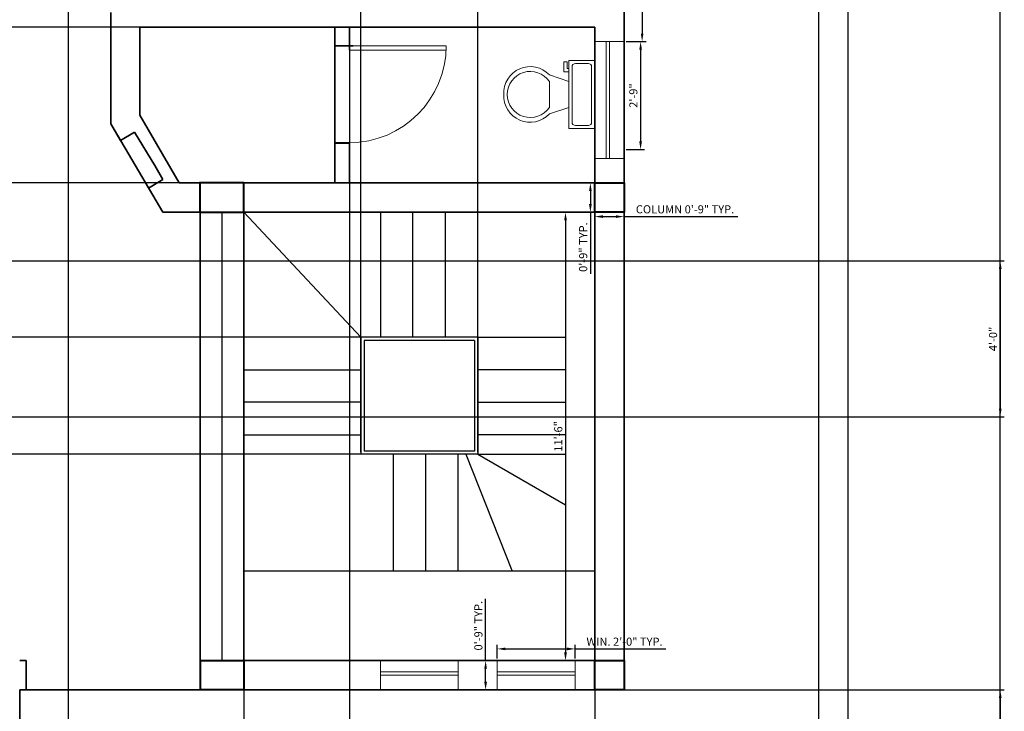
# Model space of a CAD drawing. Units: inches. Extents: x 1624 to 3956, y 1589 to 5028.
# Tile 3 of 16: x 1915 to 2218, y 1862 to 2075. Entities that reach past the tile are written whole.
import ezdxf

# ---------------------------------------------------------------- set-up
doc = ezdxf.new("R2010")
doc.units = ezdxf.units.IN
for name, color, linetype, lineweight in [('A-ANNO-DIMS', 2, 'Continuous', 13), ('A-COLS', 1, 'Continuous', 40), ('A-DOOR', 3, 'Continuous', 18), ('A-FLOR-FIXT', 9, 'Continuous', 18), ('A-FLOR-STRS', 7, 'Continuous', 25), ('A-GLAZ', 4, 'Continuous', 18), ('A-WALL', 7, 'Continuous', 35), ('C-PROP', 7, 'Continuous', 25)]:
    doc.layers.add(name, color=color, linetype=linetype, lineweight=lineweight)
doc.styles.get("Standard").update_dxf_attribs({"font": 'arial.ttf'})
doc.dimstyles.new('Copy of ISO-25', dxfattribs={"dimtxt": 2.5, "dimasz": 2.5, "dimexe": 1.25, "dimexo": 0.625, "dimtad": 1, "dimdec": 1, "dimlunit": 4, "dimtxsty": 'Standard', "dimcen": 2.5, "dimadec": 0, "dimazin": 0, "dimtfac": 1, "dimtdec": 1, "dimtmove": 0, "dimatfit": 3, "dimfxl": 1, "dimarcsym": 0})

# ---------------------------------------------------------------- blocks, each defined once
blk = doc.blocks.new('*D1')
at = {"layer": 'A-ANNO-DIMS', "color": 0, "lineweight": -2, "transparency": 16777216}
for p, q in [((2090.95, 2015.79), (2081.32, 2015.79)), ((2082.57, 2013.29), (2082.57, 1880.29)), ((2090.95, 1877.79), (2081.32, 1877.79))]:
    blk.add_line(p, q, dxfattribs=at)
at = {"layer": 'A-ANNO-DIMS', "color": 0, "transparency": 16777216}
for points in [[(2082.15, 2013.29), (2082.99, 2013.29), (2082.57, 2015.79)], [(2082.15, 1880.29), (2082.99, 1880.29), (2082.57, 1877.79)]]:
    blk.add_solid(points, dxfattribs=at)
at = {"layer": 'Defpoints', "color": 0, "transparency": 16777216}
for p in [(2091.58, 2015.79), (2082.57, 1877.79), (2091.58, 1877.79)]:
    blk.add_point(p, dxfattribs=at)
at = {"layer": 'A-ANNO-DIMS', "color": 0, "transparency": 16777216, "insert": (2080.67, 1946.79), "char_height": 2.5, "attachment_point": 5, "rotation": 90}
blk.add_mtext('11\'-6"', dxfattribs=at)
blk = doc.blocks.new('*U7')
for p, q in [((-40, 0), (-40, 6)), ((0, 0), (0, 6))]:
    blk.add_line(p, q)
blk.add_lwpolyline([(0, 0), (0, -40), (-1.75, -40), (-1.75, 0)], close=True)
blk.add_arc((0, 0), 40, 180, 270)
blk = doc.blocks.new('*U14')
for p, q in [((241.3, -152.4), (241.3, -50.8)), ((-254, -215.9), (-203.2, -215.9)), ((-254, -241.3), (-254, -215.9)), ((-203.2, -215.9), (-203.2, -203.2)), ((-177.8, -203.2), (-177.8, -241.3)), ((-101.6, -203.2), (-152.4, -355.6)), ((101.6, -203.2), (152.4, -355.6)), ((-177.8, -241.3), (-254, -241.3)), ((101.6, -355.6), (-101.6, -355.6))]:
    blk.add_line(p, q)
blk.add_lwpolyline([(266.7, -203.2), (266.7, 0), (-266.7, 0), (-266.7, -203.2)], close=True)
for points in [[(-241.3, -50.8), (-241.3, -152.4)], [(215.9, -25.4), (-215.9, -25.4)], [(-215.9, -177.8), (215.9, -177.8)]]:
    blk.add_lwpolyline(points)
for centre, radius, start, end in [((-219.075, -47.625), 22.45064, 81.8699, 188.1301), ((219.075, -47.625), 22.45064, 351.8699, 98.1301), ((-219.075, -155.575), 22.45064, 171.869898, 278.1301), ((219.075, -155.575), 22.45064, 261.8699, 8.1301), ((-12.12088, -505.93752), 205.61935, 133.01722, 273.38), ((0.94996, -504.77674), 181.02486, 124.50543, 269.7), ((-0.94742, -504.77674), 181.02486, 270.3, 55.4946), ((12.12342, -505.93752), 205.61935, 266.62, 46.9828)]:
    blk.add_arc(centre, radius, start, end)
blk = doc.blocks.new('*D41')
at = {"layer": 'A-ANNO-DIMS', "color": 0, "lineweight": -2, "transparency": 16777216}
for p, q in [((2101.2, 2104.79), (2107.41, 2104.79)), ((2106.16, 2102.29), (2106.16, 2070.79)), ((2101.2, 2068.29), (2107.41, 2068.29))]:
    blk.add_line(p, q, dxfattribs=at)
at = {"layer": 'A-ANNO-DIMS', "color": 0, "transparency": 16777216}
for points in [[(2105.74, 2102.29), (2106.57, 2102.29), (2106.16, 2104.79)], [(2105.74, 2070.79), (2106.57, 2070.79), (2106.16, 2068.29)]]:
    blk.add_solid(points, dxfattribs=at)
at = {"layer": 'Defpoints', "color": 0, "transparency": 16777216}
for p in [(2100.58, 2104.79), (2100.58, 2068.29), (2106.16, 2068.29)]:
    blk.add_point(p, dxfattribs=at)
at = {"layer": 'A-ANNO-DIMS', "color": 0, "transparency": 16777216, "insert": (2102.58, 2086.54), "char_height": 2.5, "attachment_point": 5, "rotation": 90}
blk.add_mtext('3\'-0{\\H1x;\\S1/2;}"', dxfattribs=at)
blk = doc.blocks.new('*D42')
at = {"layer": 'A-ANNO-DIMS', "color": 0, "lineweight": -2, "transparency": 16777216}
for p, q in [((2101.2, 2068.29), (2106.93, 2068.29)), ((2105.68, 2065.79), (2105.68, 2037.58)), ((2101.2, 2035.08), (2106.93, 2035.08))]:
    blk.add_line(p, q, dxfattribs=at)
at = {"layer": 'A-ANNO-DIMS', "color": 0, "transparency": 16777216}
for points in [[(2105.27, 2065.79), (2106.1, 2065.79), (2105.68, 2068.29)], [(2105.27, 2037.58), (2106.1, 2037.58), (2105.68, 2035.08)]]:
    blk.add_solid(points, dxfattribs=at)
at = {"layer": 'Defpoints', "color": 0, "transparency": 16777216}
for p in [(2100.58, 2068.29), (2100.58, 2035.08), (2105.68, 2035.08)]:
    blk.add_point(p, dxfattribs=at)
at = {"layer": 'A-ANNO-DIMS', "color": 0, "transparency": 16777216, "insert": (2103.78, 2051.69), "char_height": 2.5, "attachment_point": 5, "rotation": 90}
blk.add_mtext('2\'-9"', dxfattribs=at)
blk = doc.blocks.new('COLUMN-9x9')
for p, q in [((0, 0), (0, 9)), ((0, 9), (9, 9)), ((9, 9), (9, 0)), ((9, 0), (0, 0))]:
    blk.add_line(p, q)
blk = doc.blocks.new('WINDOW-36IN')
for p, q in [((0, 0), (0, 9)), ((36, 9), (36, 0)), ((0, 4.5), (36, 4.5)), ((0, 3.5), (36, 3.5))]:
    blk.add_line(p, q)
blk = doc.blocks.new('WINDOW-24IN')
for p, q in [((0, 0), (0, 9)), ((24, 9), (24, 0)), ((24, 5.5), (0, 5.5)), ((24, 4.5), (0, 4.5))]:
    blk.add_line(p, q)
blk = doc.blocks.new('*D48')
at = {"layer": 'A-ANNO-DIMS', "color": 0, "lineweight": -2, "transparency": 16777216}
for p, q in [((2091.58, 2015.17), (2091.58, 2013.19)), ((2094.08, 2014.44), (2098.08, 2014.44)), ((2100.58, 2015.17), (2100.58, 2013.19)), ((2100.58, 2014.44), (2135.64, 2014.44))]:
    blk.add_line(p, q, dxfattribs=at)
at = {"layer": 'A-ANNO-DIMS', "color": 0, "transparency": 16777216}
for points in [[(2094.08, 2014.86), (2094.08, 2014.03), (2091.58, 2014.44)], [(2098.08, 2014.86), (2098.08, 2014.03), (2100.58, 2014.44)]]:
    blk.add_solid(points, dxfattribs=at)
at = {"layer": 'Defpoints', "color": 0, "transparency": 16777216}
for p in [(2091.58, 2015.79), (2100.58, 2015.79), (2100.58, 2014.44)]:
    blk.add_point(p, dxfattribs=at)
at = {"layer": 'A-ANNO-DIMS', "color": 0, "transparency": 16777216, "insert": (2119.36, 2016.36), "char_height": 2.5, "attachment_point": 5}
blk.add_mtext('COLUMN 0\'-9" TYP.', dxfattribs=at)
blk = doc.blocks.new('*D49')
at = {"layer": 'A-ANNO-DIMS', "color": 0, "lineweight": -2, "transparency": 16777216}
for p, q in [((2090.95, 2024.79), (2088.98, 2024.79)), ((2090.23, 2022.29), (2090.23, 2018.29)), ((2090.95, 2015.79), (2088.98, 2015.79)), ((2090.23, 2015.79), (2090.23, 1996.81))]:
    blk.add_line(p, q, dxfattribs=at)
at = {"layer": 'A-ANNO-DIMS', "color": 0, "transparency": 16777216}
for points in [[(2089.81, 2022.29), (2090.65, 2022.29), (2090.23, 2024.79)], [(2089.81, 2018.29), (2090.65, 2018.29), (2090.23, 2015.79)]]:
    blk.add_solid(points, dxfattribs=at)
at = {"layer": 'Defpoints', "color": 0, "transparency": 16777216}
for p in [(2091.58, 2024.79), (2090.23, 2015.79), (2091.58, 2015.79)]:
    blk.add_point(p, dxfattribs=at)
at = {"layer": 'A-ANNO-DIMS', "color": 0, "transparency": 16777216, "insert": (2088.33, 2005.05), "char_height": 2.5, "attachment_point": 5, "rotation": 90}
blk.add_mtext('0\'-9" TYP.', dxfattribs=at)
blk = doc.blocks.new('*D50')
at = {"layer": 'A-ANNO-DIMS', "color": 0, "lineweight": -2, "transparency": 16777216}
for p, q in [((2061.58, 1878.42), (2061.58, 1882.64)), ((2085.58, 1878.42), (2085.58, 1882.64)), ((2064.08, 1881.39), (2083.08, 1881.39)), ((2085.58, 1881.39), (2113.4, 1881.39))]:
    blk.add_line(p, q, dxfattribs=at)
at = {"layer": 'A-ANNO-DIMS', "color": 0, "transparency": 16777216}
for points in [[(2064.08, 1881.81), (2064.08, 1880.98), (2061.58, 1881.39)], [(2083.08, 1881.81), (2083.08, 1880.98), (2085.58, 1881.39)]]:
    blk.add_solid(points, dxfattribs=at)
at = {"layer": 'Defpoints', "color": 0, "transparency": 16777216}
for p in [(2085.58, 1881.39), (2061.58, 1877.79), (2085.58, 1877.79)]:
    blk.add_point(p, dxfattribs=at)
at = {"layer": 'A-ANNO-DIMS', "color": 0, "transparency": 16777216, "insert": (2100.74, 1883.3), "char_height": 2.5, "attachment_point": 5}
blk.add_mtext('WIN. 2\'-0" TYP.', dxfattribs=at)
blk = doc.blocks.new('*D51')
at = {"layer": 'A-ANNO-DIMS', "color": 0, "lineweight": -2, "transparency": 16777216}
for p, q in [((2057.98, 1877.79), (2057.98, 1896.78)), ((2060.95, 1877.79), (2056.73, 1877.79)), ((2057.98, 1871.29), (2057.98, 1875.29)), ((2060.95, 1868.79), (2056.73, 1868.79))]:
    blk.add_line(p, q, dxfattribs=at)
at = {"layer": 'A-ANNO-DIMS', "color": 0, "transparency": 16777216}
for points in [[(2057.56, 1875.29), (2058.4, 1875.29), (2057.98, 1877.79)], [(2057.56, 1871.29), (2058.4, 1871.29), (2057.98, 1868.79)]]:
    blk.add_solid(points, dxfattribs=at)
at = {"layer": 'Defpoints', "color": 0, "transparency": 16777216}
for p in [(2057.98, 1877.79), (2061.58, 1877.79), (2061.58, 1868.79)]:
    blk.add_point(p, dxfattribs=at)
at = {"layer": 'A-ANNO-DIMS', "color": 0, "transparency": 16777216, "insert": (2056.08, 1888.54), "char_height": 2.5, "attachment_point": 5, "rotation": 90}
blk.add_mtext('0\'-9" TYP.', dxfattribs=at)
blk = doc.blocks.new('*D67')
at = {"layer": 'A-ANNO-DIMS', "color": 0, "lineweight": -2, "transparency": 16777216}
for p, q in [((2170.2, 2564.79), (2217.63, 2564.79)), ((2216.38, 1649.29), (2216.38, 2562.29)), ((2170.2, 1646.79), (2217.63, 1646.79))]:
    blk.add_line(p, q, dxfattribs=at)
at = {"layer": 'A-ANNO-DIMS', "color": 0, "transparency": 16777216}
for points in [[(2215.96, 2562.29), (2216.8, 2562.29), (2216.38, 2564.79)], [(2215.96, 1649.29), (2216.8, 1649.29), (2216.38, 1646.79)]]:
    blk.add_solid(points, dxfattribs=at)
at = {"layer": 'Defpoints', "color": 0, "transparency": 16777216}
for p in [(2169.58, 2564.79), (2216.38, 2564.79), (2169.58, 1646.79)]:
    blk.add_point(p, dxfattribs=at)
at = {"layer": 'A-ANNO-DIMS', "color": 0, "transparency": 16777216, "insert": (2214.48, 2105.79), "char_height": 2.5, "attachment_point": 5, "rotation": 90}
blk.add_mtext('76\'-6"', dxfattribs=at)
blk = doc.blocks.new('*D74')
at = {"layer": 'A-ANNO-DIMS', "color": 0, "lineweight": -2, "transparency": 16777216}
for p, q in [((1915.2, 1868.79), (2217.63, 1868.79)), ((2216.38, 1866.29), (2216.38, 1775.29)), ((1915.2, 1772.79), (2217.63, 1772.79))]:
    blk.add_line(p, q, dxfattribs=at)
at = {"layer": 'A-ANNO-DIMS', "color": 0, "transparency": 16777216}
for points in [[(2215.96, 1866.29), (2216.8, 1866.29), (2216.38, 1868.79)], [(2215.96, 1775.29), (2216.8, 1775.29), (2216.38, 1772.79)]]:
    blk.add_solid(points, dxfattribs=at)
at = {"layer": 'Defpoints', "color": 0, "transparency": 16777216}
for p in [(1914.58, 1868.79), (1914.58, 1772.79), (2216.38, 1772.79)]:
    blk.add_point(p, dxfattribs=at)
at = {"layer": 'A-ANNO-DIMS', "color": 0, "transparency": 16777216, "insert": (2214.48, 1820.79), "char_height": 2.5, "attachment_point": 5, "rotation": 90}
blk.add_mtext('8\'-0"', dxfattribs=at)
blk = doc.blocks.new('*D85')
at = {"layer": 'A-ANNO-DIMS', "color": 0, "lineweight": -2, "transparency": 16777216}
for p, q in [((1983.58, 1877.17), (1983.58, 1589.9)), ((2091.58, 1877.17), (2091.58, 1589.9)), ((2089.08, 1591.15), (1986.08, 1591.15))]:
    blk.add_line(p, q, dxfattribs=at)
at = {"layer": 'A-ANNO-DIMS', "color": 0, "transparency": 16777216}
for points in [[(1986.08, 1591.57), (1986.08, 1590.73), (1983.58, 1591.15)], [(2089.08, 1591.57), (2089.08, 1590.73), (2091.58, 1591.15)]]:
    blk.add_solid(points, dxfattribs=at)
at = {"layer": 'Defpoints', "color": 0, "transparency": 16777216}
for p in [(1983.58, 1877.79), (2091.58, 1877.79), (1983.58, 1591.15)]:
    blk.add_point(p, dxfattribs=at)
at = {"layer": 'A-ANNO-DIMS', "color": 0, "transparency": 16777216, "insert": (2037.58, 1593.05), "char_height": 2.5, "attachment_point": 5}
blk.add_mtext('9\'-0"', dxfattribs=at)
blk = doc.blocks.new('*D87')
at = {"layer": 'A-ANNO-DIMS', "color": 0, "lineweight": -2, "transparency": 16777216}
for p, q in [((1737.64, 2000.79), (2217.63, 2000.79)), ((2216.38, 1998.29), (2216.38, 1955.29)), ((1737.64, 1952.79), (2217.63, 1952.79))]:
    blk.add_line(p, q, dxfattribs=at)
at = {"layer": 'A-ANNO-DIMS', "color": 0, "transparency": 16777216}
for points in [[(2215.96, 1998.29), (2216.8, 1998.29), (2216.38, 2000.79)], [(2215.96, 1955.29), (2216.8, 1955.29), (2216.38, 1952.79)]]:
    blk.add_solid(points, dxfattribs=at)
at = {"layer": 'Defpoints', "color": 0, "transparency": 16777216}
for p in [(1737.01, 2000.79), (1737.01, 1952.79), (2216.38, 1952.79)]:
    blk.add_point(p, dxfattribs=at)
at = {"layer": 'A-ANNO-DIMS', "color": 0, "transparency": 16777216, "insert": (2214.48, 1976.79), "char_height": 2.5, "attachment_point": 5, "rotation": 90}
blk.add_mtext('4\'-0"', dxfattribs=at)
blk = doc.blocks.new('*D90')
at = {"layer": 'A-ANNO-DIMS', "color": 0, "lineweight": -2, "transparency": 16777216}
for p, q in [((2019.58, 1941.92), (2019.58, 2612.84)), ((2055.58, 1941.92), (2055.58, 2612.84)), ((2022.08, 2611.59), (2053.08, 2611.59))]:
    blk.add_line(p, q, dxfattribs=at)
at = {"layer": 'A-ANNO-DIMS', "color": 0, "transparency": 16777216}
for points in [[(2022.08, 2612.01), (2022.08, 2611.18), (2019.58, 2611.59)], [(2053.08, 2612.01), (2053.08, 2611.18), (2055.58, 2611.59)]]:
    blk.add_solid(points, dxfattribs=at)
at = {"layer": 'Defpoints', "color": 0, "transparency": 16777216}
for p in [(2055.58, 2611.59), (2019.58, 1941.29), (2055.58, 1941.29)]:
    blk.add_point(p, dxfattribs=at)
at = {"layer": 'A-ANNO-DIMS', "color": 0, "transparency": 16777216, "insert": (2037.58, 2613.5), "char_height": 2.5, "attachment_point": 5}
blk.add_mtext('3\'-0"', dxfattribs=at)
blk = doc.blocks.new('*D91')
at = {"layer": 'A-ANNO-DIMS', "color": 0, "lineweight": -2, "transparency": 16777216}
for p, q in [((2054.95, 1977.29), (1628.86, 1977.29)), ((1630.11, 1943.79), (1630.11, 1974.79)), ((2054.95, 1941.29), (1628.86, 1941.29))]:
    blk.add_line(p, q, dxfattribs=at)
at = {"layer": 'A-ANNO-DIMS', "color": 0, "transparency": 16777216}
for points in [[(1629.69, 1974.79), (1630.53, 1974.79), (1630.11, 1977.29)], [(1629.69, 1943.79), (1630.53, 1943.79), (1630.11, 1941.29)]]:
    blk.add_solid(points, dxfattribs=at)
at = {"layer": 'Defpoints', "color": 0, "transparency": 16777216}
for p in [(1630.11, 1977.29), (2055.58, 1977.29), (2055.58, 1941.29)]:
    blk.add_point(p, dxfattribs=at)
at = {"layer": 'A-ANNO-DIMS', "color": 0, "transparency": 16777216, "insert": (1628.21, 1959.29), "char_height": 2.5, "attachment_point": 5, "rotation": 90}
blk.add_mtext('3\'-0"', dxfattribs=at)
blk = doc.blocks.new('*D92')
at = {"layer": 'A-ANNO-DIMS', "color": 0, "lineweight": -2, "transparency": 16777216}
for p, q in [((2016.08, 2072.17), (2016.08, 1589.9)), ((2091.58, 2072.17), (2091.58, 1589.9)), ((2018.58, 1591.15), (2089.08, 1591.15))]:
    blk.add_line(p, q, dxfattribs=at)
at = {"layer": 'A-ANNO-DIMS', "color": 0, "transparency": 16777216}
for points in [[(2018.58, 1591.57), (2018.58, 1590.73), (2016.08, 1591.15)], [(2089.08, 1591.57), (2089.08, 1590.73), (2091.58, 1591.15)]]:
    blk.add_solid(points, dxfattribs=at)
at = {"layer": 'Defpoints', "color": 0, "transparency": 16777216}
for p in [(2016.08, 2072.79), (2091.58, 2072.79), (2091.58, 1591.15)]:
    blk.add_point(p, dxfattribs=at)
at = {"layer": 'A-ANNO-DIMS', "color": 0, "transparency": 16777216, "insert": (2053.83, 1593.07), "char_height": 2.5, "attachment_point": 5}
blk.add_mtext('6\'-3 1/2"', dxfattribs=at)
blk = doc.blocks.new('*D93')
at = {"layer": 'A-ANNO-DIMS', "color": 0, "lineweight": -2, "transparency": 16777216}
for p, q in [((2090.95, 2072.79), (1628.86, 2072.79)), ((1630.11, 2070.29), (1630.11, 2027.29)), ((2090.95, 2024.79), (1628.86, 2024.79))]:
    blk.add_line(p, q, dxfattribs=at)
at = {"layer": 'A-ANNO-DIMS', "color": 0, "transparency": 16777216}
for points in [[(1629.69, 2070.29), (1630.53, 2070.29), (1630.11, 2072.79)], [(1629.69, 2027.29), (1630.53, 2027.29), (1630.11, 2024.79)]]:
    blk.add_solid(points, dxfattribs=at)
at = {"layer": 'Defpoints', "color": 0, "transparency": 16777216}
for p in [(2091.58, 2072.79), (1630.11, 2024.79), (2091.58, 2024.79)]:
    blk.add_point(p, dxfattribs=at)
at = {"layer": 'A-ANNO-DIMS', "color": 0, "transparency": 16777216, "insert": (1628.21, 2048.79), "char_height": 2.5, "attachment_point": 5, "rotation": 90}
blk.add_mtext('4\'-0"', dxfattribs=at)
blk = doc.blocks.new('*D94')
at = {"layer": 'A-ANNO-DIMS', "color": 0, "lineweight": -2, "transparency": 16777216}
for p, q in [((1893.52, 2315.17), (1893.52, 1589.9)), ((1929.52, 2315.17), (1929.52, 1589.9)), ((1896.02, 1591.15), (1927.02, 1591.15))]:
    blk.add_line(p, q, dxfattribs=at)
at = {"layer": 'A-ANNO-DIMS', "color": 0, "transparency": 16777216}
for points in [[(1896.02, 1591.57), (1896.02, 1590.73), (1893.52, 1591.15)], [(1927.02, 1591.57), (1927.02, 1590.73), (1929.52, 1591.15)]]:
    blk.add_solid(points, dxfattribs=at)
at = {"layer": 'Defpoints', "color": 0, "transparency": 16777216}
for p in [(1893.52, 2315.79), (1929.52, 2315.79), (1929.52, 1591.15)]:
    blk.add_point(p, dxfattribs=at)
at = {"layer": 'A-ANNO-DIMS', "color": 0, "transparency": 16777216, "insert": (1911.52, 1593.05), "char_height": 2.5, "attachment_point": 5}
blk.add_mtext('3\'-0"', dxfattribs=at)

msp = doc.modelspace()

# ---------------------------------------------------------------- linework, layer by layer
at = {"layer": 'A-COLS'}
for p, q in [((1983.58, 2024.79), (1969.89, 2024.79)), ((1970.08, 2015.79), (1970.08, 2024.79)), ((1983.58, 2015.79), (1983.58, 2024.79)), ((1970.08, 2015.79), (1983.58, 2015.79)), ((1970.08, 1877.79), (1983.58, 1877.79)), ((1970.08, 1877.79), (1970.08, 1868.79)), ((1983.58, 1877.79), (1983.58, 1868.79)), ((1983.58, 1868.79), (1970.08, 1868.79))]:
    msp.add_line(p, q, dxfattribs=at)
at = {"layer": 'A-FLOR-STRS'}
for p, q in [((1976.83, 2015.79), (1976.83, 1877.79)), ((2019.58, 1977.29), (1983.58, 2015.79)), ((2035.58, 2015.79), (2025.58, 2015.79)), ((2025.58, 2015.79), (2025.58, 1977.29)), ((2035.58, 1977.29), (2035.58, 2015.79)), ((2055.58, 2015.79), (2045.58, 2015.79)), ((2045.58, 2015.79), (2045.58, 1977.29)), ((2055.58, 1977.29), (2055.58, 2015.79)), ((2091.58, 2015.79), (2091.58, 1905.29)), ((2019.58, 1977.29), (1983.58, 1977.29)), ((1983.58, 1977.29), (1983.58, 1967.29)), ((2055.58, 1977.29), (2019.58, 1977.29)), ((2019.58, 1977.29), (2019.58, 1941.29)), ((2020.58, 1976.29), (2020.58, 1942.29)), ((2054.58, 1976.29), (2020.58, 1976.29)), ((2045.58, 1977.29), (2035.58, 1977.29)), ((2054.58, 1976.29), (2054.58, 1942.29)), ((2055.58, 1977.29), (2055.58, 1941.29)), ((2055.58, 1977.29), (2082.57, 1977.29)), ((2082.57, 1977.29), (2082.57, 1967.29)), ((1983.58, 1967.29), (2019.58, 1967.29)), ((2019.58, 1967.29), (2019.58, 1957.29)), ((2082.57, 1967.29), (2055.58, 1967.29)), ((2055.58, 1967.29), (2055.58, 1957.29)), ((2019.58, 1957.29), (1983.58, 1957.29)), ((1983.58, 1957.29), (1983.58, 1947.29)), ((2055.58, 1957.29), (2082.57, 1957.29)), ((2082.57, 1957.29), (2082.57, 1947.29)), ((1983.58, 1947.29), (2019.58, 1947.29)), ((2019.58, 1947.29), (2019.58, 1941.29)), ((2082.57, 1947.29), (2055.58, 1947.29)), ((2019.58, 1941.29), (1983.58, 1941.29)), ((2055.58, 1941.29), (2019.58, 1941.29)), ((2054.58, 1942.29), (2020.58, 1942.29)), ((2029.58, 1905.29), (2029.58, 1941.29)), ((2039.58, 1905.29), (2039.58, 1941.29)), ((2049.58, 1905.29), (2049.58, 1941.29)), ((2051.87, 1941.29), (2066.13, 1905.29)), ((2055.58, 1941.29), (2082.57, 1941.29)), ((2055.58, 1941.29), (2082.57, 1925.75)), ((2091.58, 1923.79), (2091.58, 1933.79)), ((2091.58, 1905.29), (1983.58, 1905.29)), ((2039.58, 1877.79), (2039.58, 1877.79))]:
    msp.add_line(p, q, dxfattribs=at)
at = {"layer": 'A-GLAZ'}
for p, q in [((2100.58, 2068.29), (2100.58, 2032.29)), ((2049.58, 1868.79), (2025.58, 1868.79)), ((2085.58, 1868.79), (2061.58, 1868.79))]:
    msp.add_line(p, q, dxfattribs=at)
at = {"layer": 'A-WALL'}
for p, q in [((2100.58, 2161.29), (2100.58, 2033.29)), ((1942.58, 2077.29), (1942.58, 2072.79)), ((2100.58, 2077.29), (2100.58, 2072.79)), ((2100.58, 2077.29), (2100.58, 2072.79)), ((1942.58, 2072.79), (1942.58, 2042.98)), ((2091.58, 2072.79), (1951.58, 2072.79)), ((1951.58, 2072.79), (1951.58, 2047.33)), ((2011.58, 2024.79), (2011.58, 2072.79)), ((2016.08, 2072.79), (2016.08, 2067.01)), ((2016.08, 2065.69), (2016.08, 2072.79)), ((2091.58, 2072.79), (2091.58, 2024.79)), ((2091.58, 2072.79), (2091.58, 2068.29)), ((2100.58, 2072.79), (2100.58, 2024.79)), ((2017.21, 2067.01), (2011.58, 2067.01)), ((2011.58, 2067.01), (2011.58, 2067)), ((1951.58, 2047.33), (1951.58, 2045.69)), ((1951.58, 2045.69), (1951.58, 2045.69)), ((1951.58, 2045.69), (1963.61, 2024.79)), ((1942.58, 2042.98), (1958.62, 2015.79)), ((1942.58, 2042.98), (1945.6, 2037.85)), ((1945.6, 2037.85), (1949.91, 2040.39)), ((1949.91, 2040.39), (1956.12, 2030.12)), ((2011.58, 2037.2), (2011.58, 2037.01)), ((2011.58, 2037.01), (2016.08, 2037.01)), ((2016.08, 2024.79), (2016.08, 2037.2)), ((2100.58, 2033.29), (2100.58, 1988.29)), ((1956.12, 2030.12), (1958.67, 2025.82)), ((1958.67, 2025.82), (1954.24, 2023.21)), ((1963.61, 2024.79), (2016.08, 2024.79)), ((2091.58, 2024.79), (2016.08, 2024.79)), ((2016.08, 2024.79), (2091.58, 2024.79)), ((1970.08, 2015.79), (1958.62, 2015.79)), ((1970.08, 2015.79), (1970.08, 1877.79)), ((2016.08, 2015.79), (1983.58, 2015.79)), ((2091.58, 2015.79), (1983.58, 2015.79)), ((1983.58, 2015.79), (1983.58, 1877.79)), ((2091.58, 2015.79), (2016.08, 2015.79)), ((2091.58, 2015.79), (2091.58, 1877.79)), ((2100.58, 1988.29), (2100.58, 1877.79)), ((1914.58, 1877.79), (1914.57, 1877.79)), ((1916.58, 1877.79), (1914.58, 1877.79)), ((1914.58, 1877.79), (1916.58, 1877.79)), ((1916.58, 1877.79), (1916.58, 1868.79)), ((2091.58, 1877.79), (1983.58, 1877.79)), ((2061.58, 1877.79), (2049.58, 1877.79)), ((2091.58, 1877.79), (2085.58, 1877.79)), ((2100.58, 1877.79), (2100.58, 1868.79)), ((1914.58, 1868.79), (1914.58, 1772.79)), ((1916.58, 1868.79), (1914.58, 1868.79)), ((1916.58, 1868.79), (1970.08, 1868.79)), ((2100.58, 1868.79), (1970.08, 1868.79))]:
    msp.add_line(p, q, dxfattribs=at)
at = {"layer": 'C-PROP'}
for p, q in [((2169.58, 1652.79), (2169.58, 2559.46)), ((2160.58, 1652.79), (2160.58, 2555.79))]:
    msp.add_line(p, q, dxfattribs=at)

# ---------------------------------------------------------------- block references
at = {"layer": 'A-COLS'}
for p, rotation in [((2091.58, 2024.79), 270.0000000000029), ((2091.58, 1877.79), 270.0000000000087)]:
    msp.add_blockref('COLUMN-9x9', p, dxfattribs=dict(at, rotation=rotation))
at = {"layer": 'A-DOOR', "xscale": 0.7449753872757019, "yscale": 0.7449753872757019, "zscale": 0.7449753872757019, "rotation": 89.99999999999999}
msp.add_blockref('*U7', (2016.05, 2067), dxfattribs=at)
at = {"layer": 'A-FLOR-FIXT', "xscale": 0.0393700787401575, "yscale": 0.0393700787401575, "zscale": 0.0393700787401575, "rotation": 270}
msp.add_blockref('*U14', (2091.6, 2052.03), dxfattribs=at)
at = {"layer": 'A-GLAZ', "rotation": 270}
msp.add_blockref('WINDOW-36IN', (2091.58, 2068.29), dxfattribs=at)
at = {"layer": 'A-GLAZ'}
for p in [(2025.58, 1868.79), (2061.58, 1868.79)]:
    msp.add_blockref('WINDOW-24IN', p, dxfattribs=at)

# ---------------------------------------------------------------- dimensions: what is measured, and where the dimension line sits
at = {"layer": 'A-ANNO-DIMS'}
for base, p1, p2, picture, middle in [((2055.58, 2611.59), (2019.58, 1941.29), (2055.58, 1941.29), '*D90', (2037.58, 2613.5)), ((1929.52, 1591.15), (1893.52, 2315.79), (1929.52, 2315.79), '*D94', (1911.52, 1593.05)), ((2091.58, 1591.15), (2016.08, 2072.79), (2091.58, 2072.79), '*D92', (2053.83, 1593.07)), ((1983.58, 1591.15), (2091.58, 1877.79), (1983.58, 1877.79), '*D85', (2037.58, 1593.05))]:
    dim = msp.add_linear_dim(base=base, p1=p1, p2=p2, dimstyle='Copy of ISO-25', override={"dimdec": 1, "dimlfac": 1, "dimrnd": 0, "dimzin": 1, "dimdsep": 46, "dimlunit": 4, "dimfrac": 2}, dxfattribs=at)
    dim.commit()
    dim.dimension.update_dxf_attribs({"geometry": picture, "text_midpoint": middle})
for base, p1, p2, override, picture, middle in [((2216.38, 2564.79), (2169.58, 1646.79), (2169.58, 2564.79), {"dimdec": 1, "dimlfac": 1, "dimrnd": 0, "dimzin": 1, "dimdsep": 46, "dimlunit": 4, "dimfrac": 2}, '*D67', (2214.48, 2105.79)), ((2106.16, 2068.29), (2100.58, 2104.79), (2100.58, 2068.29), {"dimclrd": 0, "dimclre": 0, "dimclrt": 0}, '*D41', (2102.58, 2086.54)), ((1630.11, 2024.79), (2091.58, 2072.79), (2091.58, 2024.79), {"dimdec": 1, "dimlfac": 1, "dimrnd": 0, "dimzin": 1, "dimdsep": 46, "dimlunit": 4, "dimfrac": 2}, '*D93', (1628.21, 2048.79)), ((2105.68, 2035.08), (2100.58, 2068.29), (2100.58, 2035.08), {"dimclrd": 0, "dimclre": 0, "dimclrt": 0}, '*D42', (2103.78, 2051.69)), ((2082.57, 1877.79), (2091.58, 2015.79), (2091.58, 1877.79), {"dimclrd": 0, "dimclre": 0, "dimclrt": 0}, '*D1', (2080.67, 1946.79)), ((2216.38, 1952.79), (1737.01, 2000.79), (1737.01, 1952.79), {"dimdec": 1, "dimlfac": 1, "dimrnd": 0, "dimzin": 1, "dimdsep": 46, "dimlunit": 4, "dimfrac": 2}, '*D87', (2214.48, 1976.79)), ((1630.11, 1977.29), (2055.58, 1941.29), (2055.58, 1977.29), {"dimdec": 1, "dimlfac": 1, "dimrnd": 0, "dimzin": 1, "dimdsep": 46, "dimlunit": 4, "dimfrac": 2}, '*D91', (1628.21, 1959.29)), ((2216.38, 1772.79), (1914.58, 1868.79), (1914.58, 1772.79), {"dimdec": 1, "dimlfac": 1, "dimrnd": 0, "dimzin": 1, "dimdsep": 46, "dimlunit": 4, "dimfrac": 2}, '*D74', (2214.48, 1820.79))]:
    dim = msp.add_linear_dim(base=base, p1=p1, p2=p2, angle=90, dimstyle='Copy of ISO-25', override=override, dxfattribs=at)
    dim.commit()
    dim.dimension.update_dxf_attribs({"geometry": picture, "text_midpoint": middle})
for base, p1, p2, angle, text, picture, middle in [((2090.23, 2015.79), (2091.58, 2024.79), (2091.58, 2015.79), 270, '<> TYP.', '*D49', (2088.33, 2005.05)), ((2100.58, 2014.44), (2091.58, 2015.79), (2100.58, 2015.79), 0, 'COLUMN <> TYP.', '*D48', (2119.36, 2016.36)), ((2057.98, 1877.79), (2061.58, 1868.79), (2061.58, 1877.79), 90, '<> TYP.', '*D51', (2056.08, 1888.54))]:
    dim = msp.add_linear_dim(base=base, p1=p1, p2=p2, angle=angle, text=text, dimstyle='Copy of ISO-25', override={"dimdec": 1, "dimlfac": 1, "dimrnd": 0, "dimzin": 1, "dimdsep": 46, "dimlunit": 4, "dimfrac": 2}, dxfattribs=at)
    dim.commit()
    dim.dimension.update_dxf_attribs({"geometry": picture, "text_midpoint": middle})
dim = msp.add_linear_dim(base=(2085.58, 1881.39), p1=(2061.58, 1877.79), p2=(2085.58, 1877.79), text='WIN. <> TYP.', dimstyle='Copy of ISO-25', override={"dimdec": 1, "dimlfac": 1, "dimrnd": 0, "dimzin": 1, "dimdsep": 46, "dimlunit": 4, "dimfrac": 2}, dxfattribs=at)
dim.commit()
dim.dimension.update_dxf_attribs({"geometry": '*D50', "text_midpoint": (2100.74, 1883.3)})

doc.saveas('drawing.dxf')
